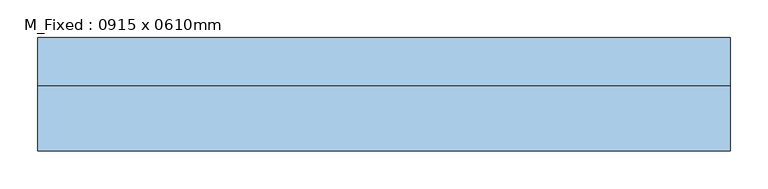
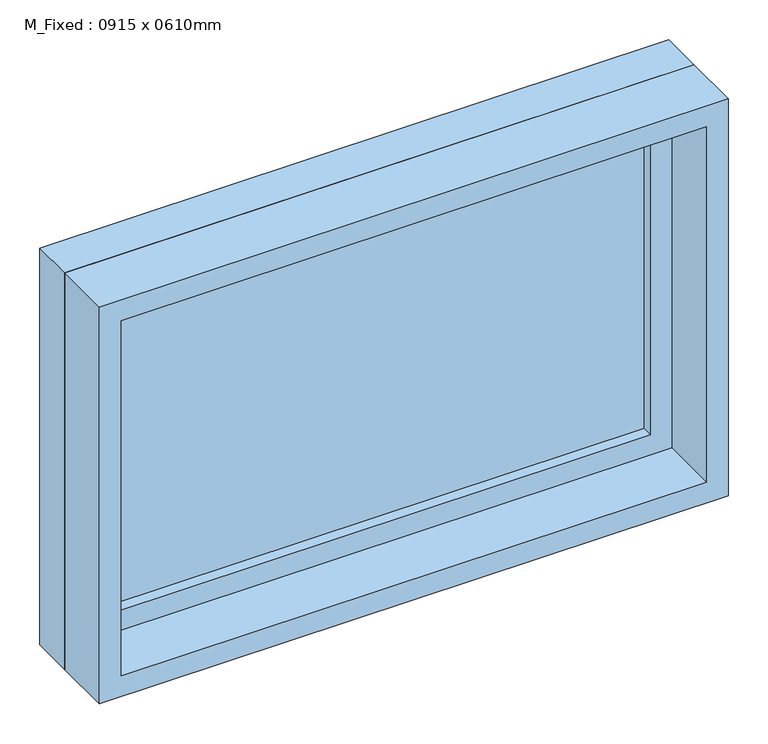
"""IFC4 building model written with IfcOpenShell, lengths in millimetres: window geometry, M_Fixed : 0915 x 0610mm."""

from ifc_helpers import new_model, si_unit, frame, origin, place, context, project, spatial, polyline, outline, extrude, source, transform, mapped, element, save


def m_fixed_0915_x_0610mm_ad787ded(model_context):
    return source(origin(), model_context, "Body", "SweptSolid", [
        extrude(outline(polyline([(-394.5, 53.0), (394.5, 53.0), (394.5, 41.0), (-394.5, 41.0), (-394.5, 53.0)])), frame((0.0, 0.0, 978.0), z_axis=(0.0, 0.0, 1.0), x_axis=(1.0, 0.0, 0.0)), (0.0, 0.0, 1.0), 484.0),
        extrude(outline(polyline([(1506.0, -438.5), (934.0, -438.5), (934.0, 438.5), (1506.0, 438.5), (1506.0, -438.5)]), holes=[polyline([(1462.0, -394.5), (1462.0, 394.5), (978.0, 394.5), (978.0, -394.5), (1462.0, -394.5)])]), frame((0.0, 25.0, 0.0), z_axis=(0.0, 1.0, 0.0), x_axis=(0.0, 0.0, 1.0)), (0.0, 0.0, 1.0), 44.0),
        extrude(outline(polyline([(1525.0, -457.5), (915.0, -457.5), (915.0, 457.5), (1525.0, 457.5), (1525.0, -457.5)]), holes=[polyline([(1506.0, -438.5), (1506.0, 438.5), (934.0, 438.5), (934.0, -438.5), (1506.0, -438.5)])]), frame((0.0, 25.0, 0.0), z_axis=(0.0, 1.0, 0.0), x_axis=(0.0, 0.0, 1.0)), (0.0, 0.0, 1.0), 63.0),
        extrude(outline(polyline([(1525.0, -457.5), (915.0, -457.5), (915.0, 457.5), (1525.0, 457.5), (1525.0, -457.5)]), holes=[polyline([(1493.0, -425.5), (1493.0, 425.5), (947.0, 425.5), (947.0, -425.5), (1493.0, -425.5)])]), frame((0.0, -62.0, 0.0), z_axis=(0.0, 1.0, 0.0), x_axis=(0.0, 0.0, 1.0)), (0.0, 0.0, 1.0), 87.0),
    ])


if __name__ == "__main__":
    model = new_model("IFC4")
    model_context = context("Model", 3, world=origin())
    ifc_project = project(units=[si_unit("LENGTHUNIT", "METRE", prefix="MILLI")], contexts=[model_context])
    site = spatial("IfcSite", under=ifc_project)
    building = spatial("IfcBuilding", under=site)
    placement = place(None, origin())
    m_fixed_0915_x_0610mm_shape = m_fixed_0915_x_0610mm_ad787ded(model_context)
    element("IfcWindow", 1, ObjectType="M_Fixed : 0915 x 0610mm", at=placement, inside=building, context=model_context, shape_type="MappedRepresentation", body=[
        mapped(m_fixed_0915_x_0610mm_shape, transform((0.0, 0.0, 0.0), x_axis=(1.0, 0.0, 0.0), y_axis=(0.0, 1.0, 0.0), z_axis=(0.0, 0.0, 1.0))),
    ])
    save(model, "model.ifc")

# Revit data of these elements
# Type "M_Fixed : 0915 x 0610mm"
#   Type Mark = "14"
#   Height = 610 mm
#   Default Sill Height = 915 mm
#   Width = 915 mm
#   Window Inset = 19 mm
#   Frame Exterior Material = Sash
#   Frame Interior Material = Sash
#   Glass Pane Material = Glass
#   Sash = Sash
#   Wall Closure = (empty or 0)
# Element 1 (IfcWindow, "M_Fixed : 0915 x 0610mm")
#   Materials on its faces: "Sash", "Glass"
# Materials
#   "Sash": class "Wood", colour RGB 136 99 55, transparency 0
#   "Glass": class "Glass", colour RGB 218 227 224, transparency 0.85, Description = "Soda Lime Glass", Cost = 0
